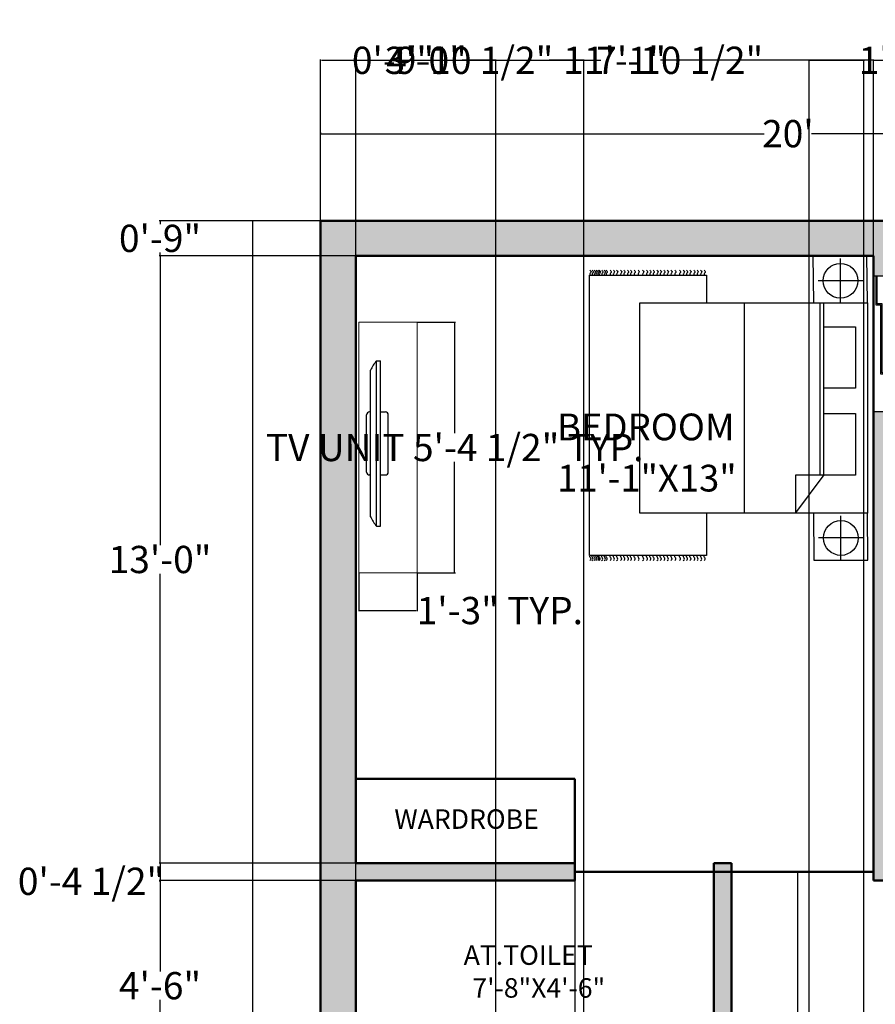
# Model space of a CAD drawing. Units: inches. Extents: x 48 to 822, y -191 to 651.
# Tile 7 of 13: x 48 to 268, y 398 to 651. Entities that reach past the tile are written whole.
import ezdxf

# ---------------------------------------------------------------- set-up
doc = ezdxf.new("R2010")
doc.units = ezdxf.units.IN
doc.header["$MEASUREMENT"] = 0
doc.layers.get('0').update_dxf_attribs({"color": 254})
for name, color, linetype, lineweight in [('A-ANNO-DIMS', 2, 'Continuous', 18), ('A-AREA-IDEN', 7, 'Continuous', 25), ('A-FURN', 8, 'Continuous', 18), ('A-GLAZ', 4, 'Continuous', 25), ('A-WALL', 7, 'Continuous', 50), ('A-WALL-PATT', 8, 'Continuous', 13)]:
    doc.layers.add(name, color=color, linetype=linetype, lineweight=lineweight)
doc.layers.add('furniture', color=250, linetype='Continuous')
doc.styles.get("Standard").update_dxf_attribs({"font": 'arial.ttf'})
doc.dimstyles.get("Standard").update_dxf_attribs({"dimtxt": 7, "dimasz": 0.18, "dimexe": 0.18, "dimexo": 0.0625, "dimgap": 0.09, "dimtad": 0, "dimtih": 1, "dimtoh": 1, "dimzin": 0, "dimdsep": 46, "dimlunit": 3, "dimtxsty": 'Standard', "dimcen": 0.09, "dimadec": 0, "dimazin": 0, "dimtfac": 1, "dimtofl": 0, "dimtmove": 0, "dimatfit": 3, "dimfxl": 1, "dimtolj": 1, "dimtzin": 0, "dimarcsym": 0})

# ---------------------------------------------------------------- blocks, each defined once
blk = doc.blocks.new('CARPET')
at = {"layer": 'furniture'}
for p, q in [((-51.53, -98.11), (-51.53, -55.12)), ((-51.53, -55.12), (-41.27, -55.12)), ((36, -55.12), (51.55, -55.12)), ((51.55, -55.12), (51.55, -98.11)), ((51.55, -98.11), (-51.53, -98.11))]:
    blk.add_line(p, q, dxfattribs=at)
for points, knots in [([(-53.37, -55.99), (-53.22, -55.8), (-52.9, -55.41), (-52.34, -55.8), (-51.89, -56.08), (-51.65, -55.91), (-51.53, -55.83)], [0, 0, 0, 0, 0.653278, 1.290138, 1.740457, 2.114451, 2.114451, 2.114451, 2.114451]), ([(-53.37, -57.26), (-53.22, -57.07), (-52.9, -56.67), (-52.34, -57.07), (-51.89, -57.35), (-51.65, -57.17), (-51.53, -57.1)], [0, 0, 0, 0, 0.653278, 1.290138, 1.740457, 2.114451, 2.114451, 2.114451, 2.114451]), ([(53.37, -55.99), (53.22, -55.8), (52.9, -55.41), (52.34, -55.8), (51.89, -56.08), (51.65, -55.91), (51.53, -55.83)], [0, 0, 0, 0, 0.653278, 1.290138, 1.740457, 2.114451, 2.114451, 2.114451, 2.114451]), ([(53.37, -57.26), (53.22, -57.07), (52.9, -56.67), (52.34, -57.07), (51.89, -57.35), (51.65, -57.17), (51.53, -57.1)], [0, 0, 0, 0, 0.653278, 1.290138, 1.740457, 2.114451, 2.114451, 2.114451, 2.114451]), ([(-53.37, -58.59), (-53.22, -58.4), (-52.9, -58.01), (-52.34, -58.4), (-51.89, -58.68), (-51.65, -58.5), (-51.53, -58.43)], [0, 0, 0, 0, 0.653278, 1.290138, 1.740457, 2.114451, 2.114451, 2.114451, 2.114451]), ([(-53.37, -59.78), (-53.22, -59.58), (-52.9, -59.19), (-52.34, -59.58), (-51.89, -59.86), (-51.65, -59.69), (-51.53, -59.61)], [0, 0, 0, 0, 0.653278, 1.290138, 1.740457, 2.114451, 2.114451, 2.114451, 2.114451]), ([(-53.37, -61.22), (-53.22, -61.02), (-52.9, -60.63), (-52.34, -61.02), (-51.89, -61.3), (-51.65, -61.13), (-51.53, -61.05)], [0, 0, 0, 0, 0.653278, 1.290138, 1.740457, 2.114451, 2.114451, 2.114451, 2.114451]), ([(53.37, -58.59), (53.22, -58.4), (52.9, -58.01), (52.34, -58.4), (51.89, -58.68), (51.65, -58.5), (51.53, -58.43)], [0, 0, 0, 0, 0.653278, 1.290138, 1.740457, 2.114451, 2.114451, 2.114451, 2.114451]), ([(53.37, -59.78), (53.22, -59.58), (52.9, -59.19), (52.34, -59.58), (51.89, -59.86), (51.65, -59.69), (51.53, -59.61)], [0, 0, 0, 0, 0.653278, 1.290138, 1.740457, 2.114451, 2.114451, 2.114451, 2.114451]), ([(53.37, -61.22), (53.22, -61.02), (52.9, -60.63), (52.34, -61.02), (51.89, -61.3), (51.65, -61.13), (51.53, -61.05)], [0, 0, 0, 0, 0.653278, 1.290138, 1.740457, 2.114451, 2.114451, 2.114451, 2.114451]), ([(-53.37, -62.44), (-53.22, -62.25), (-52.9, -61.86), (-52.34, -62.25), (-51.89, -62.53), (-51.65, -62.36), (-51.53, -62.28)], [0, 0, 0, 0, 0.653278, 1.290138, 1.740457, 2.114451, 2.114451, 2.114451, 2.114451]), ([(-53.37, -63.63), (-53.22, -63.43), (-52.9, -63.04), (-52.34, -63.43), (-51.89, -63.72), (-51.65, -63.54), (-51.53, -63.46)], [0, 0, 0, 0, 0.653278, 1.290138, 1.740457, 2.114451, 2.114451, 2.114451, 2.114451]), ([(-53.37, -65.07), (-53.22, -64.87), (-52.9, -64.48), (-52.34, -64.87), (-51.89, -65.15), (-51.65, -64.98), (-51.53, -64.9)], [0, 0, 0, 0, 0.653278, 1.290138, 1.740457, 2.114451, 2.114451, 2.114451, 2.114451]), ([(53.37, -62.44), (53.22, -62.25), (52.9, -61.86), (52.34, -62.25), (51.89, -62.53), (51.65, -62.36), (51.53, -62.28)], [0, 0, 0, 0, 0.653278, 1.290138, 1.740457, 2.114451, 2.114451, 2.114451, 2.114451]), ([(53.37, -63.63), (53.22, -63.43), (52.9, -63.04), (52.34, -63.43), (51.89, -63.72), (51.65, -63.54), (51.53, -63.46)], [0, 0, 0, 0, 0.653278, 1.290138, 1.740457, 2.114451, 2.114451, 2.114451, 2.114451]), ([(53.37, -65.07), (53.22, -64.87), (52.9, -64.48), (52.34, -64.87), (51.89, -65.15), (51.65, -64.98), (51.53, -64.9)], [0, 0, 0, 0, 0.653278, 1.290138, 1.740457, 2.114451, 2.114451, 2.114451, 2.114451]), ([(-53.37, -66.76), (-53.22, -66.56), (-52.9, -66.17), (-52.34, -66.56), (-51.89, -66.84), (-51.65, -66.67), (-51.53, -66.59)], [0, 0, 0, 0, 0.653278, 1.290138, 1.740457, 2.114451, 2.114451, 2.114451, 2.114451]), ([(-53.37, -68.2), (-53.22, -68), (-52.9, -67.61), (-52.34, -68), (-51.89, -68.28), (-51.65, -68.11), (-51.53, -68.03)], [0, 0, 0, 0, 0.653278, 1.290138, 1.740457, 2.114451, 2.114451, 2.114451, 2.114451]), ([(53.37, -66.76), (53.22, -66.56), (52.9, -66.17), (52.34, -66.56), (51.89, -66.84), (51.65, -66.67), (51.53, -66.59)], [0, 0, 0, 0, 0.653278, 1.290138, 1.740457, 2.114451, 2.114451, 2.114451, 2.114451]), ([(53.37, -68.2), (53.22, -68), (52.9, -67.61), (52.34, -68), (51.89, -68.28), (51.65, -68.11), (51.53, -68.03)], [0, 0, 0, 0, 0.653278, 1.290138, 1.740457, 2.114451, 2.114451, 2.114451, 2.114451]), ([(-53.37, -69.53), (-53.22, -69.33), (-52.9, -68.94), (-52.34, -69.33), (-51.89, -69.61), (-51.65, -69.44), (-51.53, -69.36)], [0, 0, 0, 0, 0.653278, 1.290138, 1.740457, 2.114451, 2.114451, 2.114451, 2.114451]), ([(-53.37, -70.79), (-53.22, -70.6), (-52.9, -70.21), (-52.34, -70.6), (-51.89, -70.88), (-51.65, -70.7), (-51.53, -70.63)], [0, 0, 0, 0, 0.653278, 1.290138, 1.740457, 2.114451, 2.114451, 2.114451, 2.114451]), ([(-53.37, -72.12), (-53.22, -71.93), (-52.9, -71.54), (-52.34, -71.93), (-51.89, -72.21), (-51.65, -72.04), (-51.53, -71.96)], [0, 0, 0, 0, 0.653278, 1.290138, 1.740457, 2.114451, 2.114451, 2.114451, 2.114451]), ([(53.37, -69.53), (53.22, -69.33), (52.9, -68.94), (52.34, -69.33), (51.89, -69.61), (51.65, -69.44), (51.53, -69.36)], [0, 0, 0, 0, 0.653278, 1.290138, 1.740457, 2.114451, 2.114451, 2.114451, 2.114451]), ([(53.37, -70.79), (53.22, -70.6), (52.9, -70.21), (52.34, -70.6), (51.89, -70.88), (51.65, -70.7), (51.53, -70.63)], [0, 0, 0, 0, 0.653278, 1.290138, 1.740457, 2.114451, 2.114451, 2.114451, 2.114451]), ([(53.37, -72.12), (53.22, -71.93), (52.9, -71.54), (52.34, -71.93), (51.89, -72.21), (51.65, -72.04), (51.53, -71.96)], [0, 0, 0, 0, 0.653278, 1.290138, 1.740457, 2.114451, 2.114451, 2.114451, 2.114451]), ([(-53.37, -73.31), (-53.22, -73.11), (-52.9, -72.72), (-52.34, -73.11), (-51.89, -73.4), (-51.65, -73.22), (-51.53, -73.14)], [0, 0, 0, 0, 0.653278, 1.290138, 1.740457, 2.114451, 2.114451, 2.114451, 2.114451]), ([(-53.37, -74.75), (-53.22, -74.55), (-52.9, -74.16), (-52.34, -74.55), (-51.89, -74.83), (-51.65, -74.66), (-51.53, -74.58)], [0, 0, 0, 0, 0.653278, 1.290138, 1.740457, 2.114451, 2.114451, 2.114451, 2.114451]), ([(-53.37, -75.98), (-53.22, -75.78), (-52.9, -75.39), (-52.34, -75.78), (-51.89, -76.06), (-51.65, -75.89), (-51.53, -75.81)], [0, 0, 0, 0, 0.653278, 1.290138, 1.740457, 2.114451, 2.114451, 2.114451, 2.114451]), ([(53.37, -73.31), (53.22, -73.11), (52.9, -72.72), (52.34, -73.11), (51.89, -73.4), (51.65, -73.22), (51.53, -73.14)], [0, 0, 0, 0, 0.653278, 1.290138, 1.740457, 2.114451, 2.114451, 2.114451, 2.114451]), ([(53.37, -74.75), (53.22, -74.55), (52.9, -74.16), (52.34, -74.55), (51.89, -74.83), (51.65, -74.66), (51.53, -74.58)], [0, 0, 0, 0, 0.653278, 1.290138, 1.740457, 2.114451, 2.114451, 2.114451, 2.114451]), ([(53.37, -75.98), (53.22, -75.78), (52.9, -75.39), (52.34, -75.78), (51.89, -76.06), (51.65, -75.89), (51.53, -75.81)], [0, 0, 0, 0, 0.653278, 1.290138, 1.740457, 2.114451, 2.114451, 2.114451, 2.114451]), ([(-53.37, -77.16), (-53.22, -76.96), (-52.9, -76.57), (-52.34, -76.96), (-51.89, -77.25), (-51.65, -77.07), (-51.53, -76.99)], [0, 0, 0, 0, 0.653278, 1.290138, 1.740457, 2.114451, 2.114451, 2.114451, 2.114451]), ([(-53.37, -78.6), (-53.22, -78.4), (-52.9, -78.01), (-52.34, -78.4), (-51.89, -78.68), (-51.65, -78.51), (-51.53, -78.43)], [0, 0, 0, 0, 0.653278, 1.290138, 1.740457, 2.114451, 2.114451, 2.114451, 2.114451]), ([(53.37, -77.16), (53.22, -76.96), (52.9, -76.57), (52.34, -76.96), (51.89, -77.25), (51.65, -77.07), (51.53, -76.99)], [0, 0, 0, 0, 0.653278, 1.290138, 1.740457, 2.114451, 2.114451, 2.114451, 2.114451]), ([(53.37, -78.6), (53.22, -78.4), (52.9, -78.01), (52.34, -78.4), (51.89, -78.68), (51.65, -78.51), (51.53, -78.43)], [0, 0, 0, 0, 0.653278, 1.290138, 1.740457, 2.114451, 2.114451, 2.114451, 2.114451]), ([(-53.37, -80.29), (-53.22, -80.09), (-52.9, -79.7), (-52.34, -80.09), (-51.89, -80.37), (-51.65, -80.2), (-51.53, -80.12)], [0, 0, 0, 0, 0.653278, 1.290138, 1.740457, 2.114451, 2.114451, 2.114451, 2.114451]), ([(-53.37, -81.73), (-53.22, -81.53), (-52.9, -81.14), (-52.34, -81.53), (-51.89, -81.81), (-51.65, -81.64), (-51.53, -81.56)], [0, 0, 0, 0, 0.653278, 1.290138, 1.740457, 2.114451, 2.114451, 2.114451, 2.114451]), ([(-53.37, -83.06), (-53.22, -82.86), (-52.9, -82.47), (-52.34, -82.86), (-51.89, -83.14), (-51.65, -82.97), (-51.53, -82.89)], [0, 0, 0, 0, 0.653278, 1.290138, 1.740457, 2.114451, 2.114451, 2.114451, 2.114451]), ([(53.37, -80.29), (53.22, -80.09), (52.9, -79.7), (52.34, -80.09), (51.89, -80.37), (51.65, -80.2), (51.53, -80.12)], [0, 0, 0, 0, 0.653278, 1.290138, 1.740457, 2.114451, 2.114451, 2.114451, 2.114451]), ([(53.37, -81.73), (53.22, -81.53), (52.9, -81.14), (52.34, -81.53), (51.89, -81.81), (51.65, -81.64), (51.53, -81.56)], [0, 0, 0, 0, 0.653278, 1.290138, 1.740457, 2.114451, 2.114451, 2.114451, 2.114451]), ([(53.37, -83.06), (53.22, -82.86), (52.9, -82.47), (52.34, -82.86), (51.89, -83.14), (51.65, -82.97), (51.53, -82.89)], [0, 0, 0, 0, 0.653278, 1.290138, 1.740457, 2.114451, 2.114451, 2.114451, 2.114451]), ([(-53.37, -84.18), (-53.22, -83.99), (-52.9, -83.6), (-52.34, -83.99), (-51.89, -84.27), (-51.65, -84.09), (-51.53, -84.02)], [0, 0, 0, 0, 0.653278, 1.290138, 1.740457, 2.114451, 2.114451, 2.114451, 2.114451]), ([(-53.37, -85.51), (-53.22, -85.32), (-52.9, -84.93), (-52.34, -85.32), (-51.89, -85.6), (-51.65, -85.42), (-51.53, -85.35)], [0, 0, 0, 0, 0.653278, 1.290138, 1.740457, 2.114451, 2.114451, 2.114451, 2.114451]), ([(-53.37, -86.7), (-53.22, -86.5), (-52.9, -86.11), (-52.34, -86.5), (-51.89, -86.78), (-51.65, -86.61), (-51.53, -86.53)], [0, 0, 0, 0, 0.653278, 1.290138, 1.740457, 2.114451, 2.114451, 2.114451, 2.114451]), ([(53.37, -84.18), (53.22, -83.99), (52.9, -83.6), (52.34, -83.99), (51.89, -84.27), (51.65, -84.09), (51.53, -84.02)], [0, 0, 0, 0, 0.653278, 1.290138, 1.740457, 2.114451, 2.114451, 2.114451, 2.114451]), ([(53.37, -85.51), (53.22, -85.32), (52.9, -84.93), (52.34, -85.32), (51.89, -85.6), (51.65, -85.42), (51.53, -85.35)], [0, 0, 0, 0, 0.653278, 1.290138, 1.740457, 2.114451, 2.114451, 2.114451, 2.114451]), ([(53.37, -86.7), (53.22, -86.5), (52.9, -86.11), (52.34, -86.5), (51.89, -86.78), (51.65, -86.61), (51.53, -86.53)], [0, 0, 0, 0, 0.653278, 1.290138, 1.740457, 2.114451, 2.114451, 2.114451, 2.114451]), ([(-53.37, -88.14), (-53.22, -87.94), (-52.9, -87.55), (-52.34, -87.94), (-51.89, -88.22), (-51.65, -88.05), (-51.53, -87.97)], [0, 0, 0, 0, 0.653278, 1.290138, 1.740457, 2.114451, 2.114451, 2.114451, 2.114451]), ([(-53.37, -89.36), (-53.22, -89.17), (-52.9, -88.78), (-52.34, -89.17), (-51.89, -89.45), (-51.65, -89.28), (-51.53, -89.2)], [0, 0, 0, 0, 0.653278, 1.290138, 1.740457, 2.114451, 2.114451, 2.114451, 2.114451]), ([(-53.37, -90.55), (-53.22, -90.35), (-52.9, -89.96), (-52.34, -90.35), (-51.89, -90.64), (-51.65, -90.46), (-51.53, -90.38)], [0, 0, 0, 0, 0.653278, 1.290138, 1.740457, 2.114451, 2.114451, 2.114451, 2.114451]), ([(53.37, -88.14), (53.22, -87.94), (52.9, -87.55), (52.34, -87.94), (51.89, -88.22), (51.65, -88.05), (51.53, -87.97)], [0, 0, 0, 0, 0.653278, 1.290138, 1.740457, 2.114451, 2.114451, 2.114451, 2.114451]), ([(53.37, -89.36), (53.22, -89.17), (52.9, -88.78), (52.34, -89.17), (51.89, -89.45), (51.65, -89.28), (51.53, -89.2)], [0, 0, 0, 0, 0.653278, 1.290138, 1.740457, 2.114451, 2.114451, 2.114451, 2.114451]), ([(53.37, -90.55), (53.22, -90.35), (52.9, -89.96), (52.34, -90.35), (51.9, -90.63), (51.66, -90.47), (51.55, -90.4)], [0, 0, 0, 0, 0.653278, 1.290138, 1.740457, 2.0926, 2.0926, 2.0926, 2.0926]), ([(-53.37, -91.99), (-53.22, -91.79), (-52.9, -91.4), (-52.34, -91.79), (-51.89, -92.07), (-51.65, -91.9), (-51.53, -91.82)], [0, 0, 0, 0, 0.653278, 1.290138, 1.740457, 2.114451, 2.114451, 2.114451, 2.114451]), ([(-53.37, -92.69), (-53.22, -92.48), (-52.9, -92.08), (-52.35, -92.49), (-51.89, -92.77), (-51.65, -92.6), (-51.53, -92.52)], [0, 0, 0, 0, 0.663904, 1.307406, 1.757725, 2.131719, 2.131719, 2.131719, 2.131719]), ([(-53.37, -93.61), (-53.22, -93.42), (-52.9, -93.03), (-52.34, -93.42), (-51.89, -93.7), (-51.65, -93.52), (-51.53, -93.45)], [0, 0, 0, 0, 0.653278, 1.290138, 1.740457, 2.114451, 2.114451, 2.114451, 2.114451]), ([(-53.37, -94.55), (-53.22, -94.35), (-52.9, -93.96), (-52.34, -94.35), (-51.89, -94.63), (-51.65, -94.46), (-51.53, -94.38)], [0, 0, 0, 0, 0.653278, 1.290138, 1.740457, 2.114451, 2.114451, 2.114451, 2.114451]), ([(53.37, -91.99), (53.22, -91.79), (52.9, -91.4), (52.34, -91.79), (51.9, -92.07), (51.66, -91.91), (51.55, -91.83)], [0, 0, 0, 0, 0.653278, 1.290138, 1.740457, 2.0926, 2.0926, 2.0926, 2.0926]), ([(53.37, -92.69), (53.22, -92.49), (52.9, -92.09), (52.34, -92.49), (51.9, -92.77), (51.66, -92.61), (51.55, -92.53)], [0, 0, 0, 0, 0.656792, 1.295826, 1.746145, 2.098292, 2.098292, 2.098292, 2.098292]), ([(53.37, -93.66), (53.22, -93.46), (52.9, -93.07), (52.34, -93.46), (51.9, -93.74), (51.66, -93.58), (51.55, -93.5)], [0, 0, 0, 0, 0.653278, 1.290138, 1.740457, 2.0926, 2.0926, 2.0926, 2.0926]), ([(53.37, -94.59), (53.22, -94.4), (52.9, -94.01), (52.34, -94.4), (51.9, -94.68), (51.66, -94.51), (51.55, -94.44)], [0, 0, 0, 0, 0.653278, 1.290138, 1.740457, 2.0926, 2.0926, 2.0926, 2.0926]), ([(-53.37, -95.05), (-53.22, -94.85), (-52.9, -94.46), (-52.34, -94.85), (-51.89, -95.14), (-51.65, -94.96), (-51.53, -94.88)], [0, 0, 0, 0, 0.653278, 1.290138, 1.740457, 2.114451, 2.114451, 2.114451, 2.114451]), ([(-53.37, -95.73), (-53.22, -95.54), (-52.9, -95.15), (-52.34, -95.54), (-51.89, -95.82), (-51.65, -95.65), (-51.53, -95.57)], [0, 0, 0, 0, 0.653278, 1.290138, 1.740457, 2.114451, 2.114451, 2.114451, 2.114451]), ([(-53.37, -96.38), (-53.22, -96.18), (-52.9, -95.79), (-52.34, -96.18), (-51.89, -96.47), (-51.65, -96.29), (-51.53, -96.21)], [0, 0, 0, 0, 0.653278, 1.290138, 1.740457, 2.114451, 2.114451, 2.114451, 2.114451]), ([(-53.37, -97.17), (-53.22, -96.98), (-52.9, -96.59), (-52.34, -96.98), (-51.89, -97.26), (-51.65, -97.08), (-51.53, -97.01)], [0, 0, 0, 0, 0.653278, 1.290138, 1.740457, 2.114451, 2.114451, 2.114451, 2.114451]), ([(-53.37, -97.99), (-53.22, -97.79), (-52.9, -97.4), (-52.34, -97.79), (-51.89, -98.08), (-51.65, -97.9), (-51.53, -97.82)], [0, 0, 0, 0, 0.653278, 1.290138, 1.740457, 2.114451, 2.114451, 2.114451, 2.114451]), ([(53.37, -95.78), (53.22, -95.58), (52.9, -95.19), (52.34, -95.58), (51.89, -95.86), (51.65, -95.69), (51.53, -95.61)], [0, 0, 0, 0, 0.653278, 1.290138, 1.740457, 2.114451, 2.114451, 2.114451, 2.114451]), ([(53.37, -96.43), (53.22, -96.23), (52.9, -95.84), (52.34, -96.23), (51.89, -96.51), (51.65, -96.34), (51.53, -96.26)], [0, 0, 0, 0, 0.653278, 1.290138, 1.740457, 2.114451, 2.114451, 2.114451, 2.114451]), ([(53.37, -97.22), (53.22, -97.02), (52.9, -96.63), (52.34, -97.02), (51.89, -97.3), (51.65, -97.13), (51.53, -97.05)], [0, 0, 0, 0, 0.653278, 1.290138, 1.740457, 2.114451, 2.114451, 2.114451, 2.114451]), ([(53.37, -97.99), (53.22, -97.79), (52.9, -97.4), (52.34, -97.79), (51.89, -98.08), (51.65, -97.9), (51.53, -97.82)], [0, 0, 0, 0, 0.653278, 1.290138, 1.740457, 2.114451, 2.114451, 2.114451, 2.114451]), ([(53.37, -95.1), (53.22, -94.9), (52.9, -94.51), (52.34, -94.9), (51.9, -95.18), (51.66, -95.02), (51.55, -94.94)], [0, 0, 0, 0, 0.653278, 1.290138, 1.740457, 2.0926, 2.0926, 2.0926, 2.0926])]:
    blk.add_open_spline(points, degree=3, knots=knots, dxfattribs=at)
blk = doc.blocks.new('A$C58D270C6')
at = {"layer": 'furniture'}
for p, q in [((9.09, 124.13), (9.09, 108.87)), ((1.46, 116.5), (16.73, 116.5)), ((42.08, 108), (42.08, 36)), ((14.97, 94.84), (24.62, 107.92)), ((24.62, 94.93), (24.62, 107.92)), ((14.97, 94.93), (24.62, 94.93)), ((14.97, 94.84), (14.97, 36)), ((16.22, 94.93), (16.22, 36)), ((9.25, 36), (9.25, 20.74)), ((1.62, 28.37), (16.88, 28.37))]:
    blk.add_line(p, q, dxfattribs=at)
for points in [[(18.5, 108), (18.34, 124.13), (-0.16, 124.13), (0, 108)], [(0, 108), (77.91, 108), (77.91, 36), (0, 36)], [(4.09, 94.93), (14.97, 94.93), (14.97, 73.83), (4.09, 73.83)], [(4.09, 65.23), (14.97, 65.23), (14.97, 44.13), (4.09, 44.13)], [(18.65, 19.87), (18.5, 36), (0, 36), (0.16, 19.87)]]:
    blk.add_lwpolyline(points, close=True, dxfattribs=at)
for centre in [(9.09, 116.5), (9.25, 28.37)]:
    blk.add_circle(centre, 5.95, dxfattribs=at)
at = {"layer": 'furniture', "xscale": 0.9312884925094044, "yscale": 0.9312884925094044, "zscale": 0.9312884925094044, "rotation": 90}
blk.add_blockref('CARPET', (3.79, 74.47), dxfattribs=at)
blk = doc.blocks.new('PLASMA-LARGE')
at = {"layer": 'furniture'}
for p, q in [((-7.26, 0), (7.26, 0)), ((-21, -2.5), (21, -2.5)), ((-21, -2.5), (-21, -3.5)), ((-18.61, -1), (18.61, -1)), ((-8, -1), (-8, -0.74)), ((8, -1), (8, -0.74)), ((21, -2.5), (21, -3.5)), ((-21, -3.5), (21, -3.5)), ((-8, -3.5), (-8, -4.76)), ((8, -3.5), (8, -4.76)), ((-7.26, -5.5), (7.26, -5.5))]:
    blk.add_line(p, q, dxfattribs=at)
for centre, radius, start, end in [((-7.26, -0.74), 0.744, 90, 180), ((7.26, -0.74), 0.744, 0, 90), ((-13.97, -11.05), 11.07, 114.7602, 129.4175), ((13.97, -11.05), 11.07, 50.5825, 65.2398), ((-7.26, -4.76), 0.744, 180, 270), ((7.26, -4.76), 0.744, 270, 0)]:
    blk.add_arc(centre, radius, start, end, dxfattribs=at)
blk = doc.blocks.new('*D16')
at = {"layer": 'A-ANNO-DIMS', "color": 0, "lineweight": -2, "transparency": 16777216}
for p, q in [((125.45, 622.39), (125.45, 621.91)), ((365.45, 622.39), (365.45, 621.91)), ((125.63, 622.09), (239.36, 622.09)), ((365.27, 622.09), (251.54, 622.09))]:
    blk.add_line(p, q, dxfattribs=at)
at = {"layer": 'A-ANNO-DIMS', "color": 0, "transparency": 16777216}
for points in [[(125.63, 622.12), (125.63, 622.06), (125.45, 622.09)], [(365.27, 622.12), (365.27, 622.06), (365.45, 622.09)]]:
    blk.add_solid(points, dxfattribs=at)
at = {"layer": 'Defpoints', "color": 0, "transparency": 16777216}
for p in [(125.45, 622.45), (365.45, 622.45), (365.45, 622.09)]:
    blk.add_point(p, dxfattribs=at)
at = {"layer": 'A-ANNO-DIMS', "color": 0, "transparency": 16777216, "insert": (245.45, 622.09), "char_height": 7, "attachment_point": 5}
blk.add_mtext("\\A1;20'", dxfattribs=at)
blk = doc.blocks.new('*D17')
at = {"layer": 'A-ANNO-DIMS', "color": 0, "lineweight": -2, "transparency": 16777216}
for p, q in [((109.06, 599.69), (107.79, 599.69)), ((107.97, 599.51), (107.97, 243.35)), ((107.97, -120.13), (107.97, 236.02)), ((109.06, -120.31), (107.79, -120.31))]:
    blk.add_line(p, q, dxfattribs=at)
at = {"layer": 'A-ANNO-DIMS', "color": 0, "transparency": 16777216}
for points in [[(107.94, 599.51), (108, 599.51), (107.97, 599.69)], [(107.94, -120.13), (108, -120.13), (107.97, -120.31)]]:
    blk.add_solid(points, dxfattribs=at)
at = {"layer": 'Defpoints', "color": 0, "transparency": 16777216}
for p in [(109.12, 599.69), (107.97, -120.31), (109.12, -120.31)]:
    blk.add_point(p, dxfattribs=at)
at = {"layer": 'A-ANNO-DIMS', "color": 0, "transparency": 16777216, "insert": (107.97, 239.69), "char_height": 7, "attachment_point": 5}
blk.add_mtext("\\A1;60'", dxfattribs=at)
blk = doc.blocks.new('*D20')
at = {"layer": 'A-ANNO-DIMS', "color": 0, "lineweight": -2, "transparency": 16777216}
for p, q in [((247.94, 432.26), (247.94, 367.48)), ((248, 432.44), (248.12, 432.44)), ((247.94, 295.37), (247.94, 360.15)), ((248, 295.19), (248.12, 295.19))]:
    blk.add_line(p, q, dxfattribs=at)
at = {"layer": 'A-ANNO-DIMS', "color": 0, "transparency": 16777216}
for points in [[(247.91, 432.26), (247.97, 432.26), (247.94, 432.44)], [(247.91, 295.37), (247.97, 295.37), (247.94, 295.19)]]:
    blk.add_solid(points, dxfattribs=at)
at = {"layer": 'Defpoints', "color": 0, "transparency": 16777216}
for p in [(247.94, 432.44), (247.94, 432.44), (247.94, 295.19)]:
    blk.add_point(p, dxfattribs=at)
at = {"layer": 'A-ANNO-DIMS', "color": 0, "transparency": 16777216, "insert": (247.94, 363.81), "char_height": 7, "attachment_point": 5}
blk.add_mtext('\\A1;11\'-5.25"', dxfattribs=at)
blk = doc.blocks.new('WIN-900-SLIT')
for p, q in [((271.95, 585.52), (267.45, 585.52)), ((267.45, 585.52), (267.45, 550.72)), ((268.05, 585.52), (268.05, 578.13)), ((268.38, 578.41), (268.38, 585.52)), ((271.95, 550.72), (271.95, 585.52)), ((268.05, 578.13), (269.28, 578.13)), ((269.63, 578.41), (268.38, 578.41)), ((269.28, 578.13), (269.28, 560.35)), ((269.63, 560.61), (269.63, 578.41)), ((269.28, 560.35), (270.46, 560.35)), ((270.92, 560.61), (269.63, 560.61)), ((270.46, 560.35), (270.46, 550.72)), ((270.92, 550.72), (270.92, 560.61)), ((267.45, 550.72), (271.95, 550.72))]:
    blk.add_line(p, q)
blk = doc.blocks.new('TV-UNIT')
for p, q in [((14.9, 64.44), (0, 64.44)), ((0, 64.44), (0, 0)), ((14.9, 64.44), (14.9, 0)), ((0, 0), (14.9, 0))]:
    blk.add_line(p, q)
blk = doc.blocks.new('*D38')
at = {"layer": 'A-ANNO-DIMS', "color": 0, "lineweight": -2, "transparency": 16777216}
for p, q in [((150.26, 573.68), (160.05, 573.68)), ((159.87, 573.5), (159.87, 545.17)), ((159.87, 509.42), (159.87, 537.75)), ((150.26, 509.24), (160.05, 509.24))]:
    blk.add_line(p, q, dxfattribs=at)
at = {"layer": 'A-ANNO-DIMS', "color": 0, "transparency": 16777216}
for points in [[(159.84, 573.5), (159.9, 573.5), (159.87, 573.68)], [(159.84, 509.42), (159.9, 509.42), (159.87, 509.24)]]:
    blk.add_solid(points, dxfattribs=at)
at = {"layer": 'Defpoints', "color": 0, "transparency": 16777216}
for p in [(150.2, 573.68), (159.87, 573.68), (150.2, 509.24)]:
    blk.add_point(p, dxfattribs=at)
at = {"layer": 'A-ANNO-DIMS', "color": 0, "transparency": 16777216, "insert": (159.87, 541.46), "char_height": 7, "attachment_point": 5}
blk.add_mtext('\\A1;TV UNIT 5\'-4 1/2" TYP.', dxfattribs=at)
blk = doc.blocks.new('*D39')
at = {"layer": 'A-ANNO-DIMS', "color": 0, "lineweight": -2, "transparency": 16777216}
for p, q in [((135.3, 509.17), (135.3, 499.39)), ((150.2, 509.17), (150.2, 499.39)), ((135.48, 499.57), (150.02, 499.57)), ((150.2, 499.57), (150.38, 499.57))]:
    blk.add_line(p, q, dxfattribs=at)
at = {"layer": 'A-ANNO-DIMS', "color": 0, "transparency": 16777216}
for points in [[(135.48, 499.6), (135.48, 499.54), (135.3, 499.57)], [(150.02, 499.6), (150.02, 499.54), (150.2, 499.57)]]:
    blk.add_solid(points, dxfattribs=at)
at = {"layer": 'Defpoints', "color": 0, "transparency": 16777216}
for p in [(135.3, 509.24), (150.2, 509.24), (150.2, 499.57)]:
    blk.add_point(p, dxfattribs=at)
at = {"layer": 'A-ANNO-DIMS', "color": 0, "transparency": 16777216, "insert": (171.47, 499.57), "char_height": 7, "attachment_point": 5}
blk.add_mtext('\\A1;1\'-3" TYP.', dxfattribs=at)
blk = doc.blocks.new('*D60')
at = {"layer": 'A-ANNO-DIMS', "color": 0, "lineweight": -2, "transparency": 16777216}
for p, q in [((125.45, 599.75), (125.45, 641.12)), ((125.63, 640.94), (134.27, 640.94)), ((134.45, 590.75), (134.45, 641.12)), ((134.45, 640.94), (134.63, 640.94))]:
    blk.add_line(p, q, dxfattribs=at)
at = {"layer": 'A-ANNO-DIMS', "color": 0, "transparency": 16777216}
for points in [[(125.63, 640.97), (125.63, 640.91), (125.45, 640.94)], [(134.27, 640.97), (134.27, 640.91), (134.45, 640.94)]]:
    blk.add_solid(points, dxfattribs=at)
at = {"layer": 'Defpoints', "color": 0, "transparency": 16777216}
for p in [(134.45, 640.94), (125.45, 599.69), (134.45, 590.69)]:
    blk.add_point(p, dxfattribs=at)
at = {"layer": 'A-ANNO-DIMS', "color": 0, "transparency": 16777216, "insert": (144.02, 640.94), "char_height": 7, "attachment_point": 5}
blk.add_mtext('\\A1;0\'-9"', dxfattribs=at)
blk = doc.blocks.new('*D61')
at = {"layer": 'A-ANNO-DIMS', "color": 0, "lineweight": -2, "transparency": 16777216}
for p, q in [((134.45, 590.75), (134.45, 641.12)), ((134.63, 640.94), (189.17, 640.94)), ((267.27, 640.94), (212.73, 640.94)), ((267.45, 590.75), (267.45, 641.12))]:
    blk.add_line(p, q, dxfattribs=at)
at = {"layer": 'A-ANNO-DIMS', "color": 0, "transparency": 16777216}
for points in [[(134.63, 640.97), (134.63, 640.91), (134.45, 640.94)], [(267.27, 640.97), (267.27, 640.91), (267.45, 640.94)]]:
    blk.add_solid(points, dxfattribs=at)
at = {"layer": 'Defpoints', "color": 0, "transparency": 16777216}
for p in [(267.45, 640.94), (134.45, 590.69), (267.45, 590.69)]:
    blk.add_point(p, dxfattribs=at)
at = {"layer": 'A-ANNO-DIMS', "color": 0, "transparency": 16777216, "insert": (200.95, 640.94), "char_height": 7, "attachment_point": 5}
blk.add_mtext('\\A1;11\'-1"', dxfattribs=at)
blk = doc.blocks.new('*D62')
at = {"layer": 'A-ANNO-DIMS', "color": 0, "lineweight": -2, "transparency": 16777216}
for p, q in [((267.45, 590.75), (267.45, 641.12)), ((267.63, 640.94), (271.77, 640.94)), ((271.95, 590.75), (271.95, 641.12)), ((271.95, 640.94), (272.13, 640.94))]:
    blk.add_line(p, q, dxfattribs=at)
at = {"layer": 'A-ANNO-DIMS', "color": 0, "transparency": 16777216}
for points in [[(267.63, 640.97), (267.63, 640.91), (267.45, 640.94)], [(271.77, 640.97), (271.77, 640.91), (271.95, 640.94)]]:
    blk.add_solid(points, dxfattribs=at)
at = {"layer": 'Defpoints', "color": 0, "transparency": 16777216}
for p in [(271.95, 640.94), (267.45, 590.69), (271.95, 590.69)]:
    blk.add_point(p, dxfattribs=at)
at = {"layer": 'A-ANNO-DIMS', "color": 0, "transparency": 16777216, "insert": (289.68, 640.94), "char_height": 7, "attachment_point": 5}
blk.add_mtext('\\A1;0\'-4 1/2"', dxfattribs=at)
blk = doc.blocks.new('*D70')
at = {"layer": 'A-ANNO-DIMS', "color": 0, "lineweight": -2, "transparency": 16777216}
for p, q in [((125.39, 599.69), (84.02, 599.69)), ((84.2, 599.51), (84.2, 598.85)), ((134.39, 590.69), (84.02, 590.69)), ((84.2, 590.87), (84.2, 591.52))]:
    blk.add_line(p, q, dxfattribs=at)
at = {"layer": 'A-ANNO-DIMS', "color": 0, "transparency": 16777216}
for points in [[(84.17, 599.51), (84.23, 599.51), (84.2, 599.69)], [(84.17, 590.87), (84.23, 590.87), (84.2, 590.69)]]:
    blk.add_solid(points, dxfattribs=at)
at = {"layer": 'Defpoints', "color": 0, "transparency": 16777216}
for p in [(125.45, 599.69), (84.2, 590.69), (134.45, 590.69)]:
    blk.add_point(p, dxfattribs=at)
at = {"layer": 'A-ANNO-DIMS', "color": 0, "transparency": 16777216, "insert": (84.2, 595.19), "char_height": 7, "attachment_point": 5}
blk.add_mtext('\\A1;0\'-9"', dxfattribs=at)
blk = doc.blocks.new('*D71')
at = {"layer": 'A-ANNO-DIMS', "color": 0, "lineweight": -2, "transparency": 16777216}
for p, q in [((134.39, 590.69), (84.02, 590.69)), ((84.2, 590.51), (84.2, 516.35)), ((84.2, 434.87), (84.2, 509.02)), ((134.39, 434.69), (84.02, 434.69))]:
    blk.add_line(p, q, dxfattribs=at)
at = {"layer": 'A-ANNO-DIMS', "color": 0, "transparency": 16777216}
for points in [[(84.17, 590.51), (84.23, 590.51), (84.2, 590.69)], [(84.17, 434.87), (84.23, 434.87), (84.2, 434.69)]]:
    blk.add_solid(points, dxfattribs=at)
at = {"layer": 'Defpoints', "color": 0, "transparency": 16777216}
for p in [(134.45, 590.69), (84.2, 434.69), (134.45, 434.69)]:
    blk.add_point(p, dxfattribs=at)
at = {"layer": 'A-ANNO-DIMS', "color": 0, "transparency": 16777216, "insert": (84.2, 512.69), "char_height": 7, "attachment_point": 5}
blk.add_mtext('\\A1;13\'-0"', dxfattribs=at)
blk = doc.blocks.new('*D72')
at = {"layer": 'A-ANNO-DIMS', "color": 0, "lineweight": -2, "transparency": 16777216}
for p, q in [((134.39, 434.69), (84.02, 434.69)), ((84.2, 434.51), (84.2, 430.37)), ((134.39, 430.19), (84.02, 430.19)), ((84.2, 430.19), (84.2, 430.01)), ((84.2, 430.01), (84.02, 430.01))]:
    blk.add_line(p, q, dxfattribs=at)
at = {"layer": 'A-ANNO-DIMS', "color": 0, "transparency": 16777216}
for points in [[(84.17, 434.51), (84.23, 434.51), (84.2, 434.69)], [(84.17, 430.37), (84.23, 430.37), (84.2, 430.19)]]:
    blk.add_solid(points, dxfattribs=at)
at = {"layer": 'Defpoints', "color": 0, "transparency": 16777216}
for p in [(134.45, 434.69), (84.2, 430.19), (134.45, 430.19)]:
    blk.add_point(p, dxfattribs=at)
at = {"layer": 'A-ANNO-DIMS', "color": 0, "transparency": 16777216, "insert": (66.47, 430.01), "char_height": 7, "attachment_point": 5}
blk.add_mtext('\\A1;0\'-4 1/2"', dxfattribs=at)
blk = doc.blocks.new('*D73')
at = {"layer": 'A-ANNO-DIMS', "color": 0, "lineweight": -2, "transparency": 16777216}
for p, q in [((134.39, 430.19), (84.02, 430.19)), ((84.2, 430.01), (84.2, 406.85)), ((84.2, 376.37), (84.2, 399.52)), ((134.39, 376.19), (84.02, 376.19))]:
    blk.add_line(p, q, dxfattribs=at)
at = {"layer": 'A-ANNO-DIMS', "color": 0, "transparency": 16777216}
for points in [[(84.17, 430.01), (84.23, 430.01), (84.2, 430.19)], [(84.17, 376.37), (84.23, 376.37), (84.2, 376.19)]]:
    blk.add_solid(points, dxfattribs=at)
at = {"layer": 'Defpoints', "color": 0, "transparency": 16777216}
for p in [(134.45, 430.19), (84.2, 376.19), (134.45, 376.19)]:
    blk.add_point(p, dxfattribs=at)
at = {"layer": 'A-ANNO-DIMS', "color": 0, "transparency": 16777216, "insert": (84.2, 403.19), "char_height": 7, "attachment_point": 5}
blk.add_mtext('\\A1;4\'-6"', dxfattribs=at)
blk = doc.blocks.new('*D89')
at = {"layer": 'A-ANNO-DIMS', "color": 0, "lineweight": -2, "transparency": 16777216}
for p, q in [((134.45, 295.25), (134.45, 641.12)), ((134.63, 640.94), (143.04, 640.94)), ((170.23, 640.94), (161.82, 640.94)), ((170.41, 295.25), (170.41, 641.12))]:
    blk.add_line(p, q, dxfattribs=at)
at = {"layer": 'A-ANNO-DIMS', "color": 0, "transparency": 16777216}
for points in [[(134.63, 640.97), (134.63, 640.91), (134.45, 640.94)], [(170.23, 640.97), (170.23, 640.91), (170.41, 640.94)]]:
    blk.add_solid(points, dxfattribs=at)
at = {"layer": 'Defpoints', "color": 0, "transparency": 16777216}
for p in [(170.41, 640.94), (134.45, 295.19), (170.41, 295.19)]:
    blk.add_point(p, dxfattribs=at)
at = {"layer": 'A-ANNO-DIMS', "color": 0, "transparency": 16777216, "insert": (152.43, 640.94), "char_height": 7, "attachment_point": 5}
blk.add_mtext('\\A1;3\'-0"', dxfattribs=at)
blk = doc.blocks.new('*D90')
at = {"layer": 'A-ANNO-DIMS', "color": 0, "lineweight": -2, "transparency": 16777216}
for p, q in [((250.94, 295.25), (250.94, 641.12)), ((251.12, 640.94), (264.75, 640.94)), ((264.93, 295.25), (264.93, 641.12)), ((264.93, 640.94), (265.11, 640.94))]:
    blk.add_line(p, q, dxfattribs=at)
at = {"layer": 'A-ANNO-DIMS', "color": 0, "transparency": 16777216}
for points in [[(251.12, 640.97), (251.12, 640.91), (250.94, 640.94)], [(264.75, 640.97), (264.75, 640.91), (264.93, 640.94)]]:
    blk.add_solid(points, dxfattribs=at)
at = {"layer": 'Defpoints', "color": 0, "transparency": 16777216}
for p in [(264.93, 640.94), (250.94, 295.19), (264.93, 295.19)]:
    blk.add_point(p, dxfattribs=at)
at = {"layer": 'A-ANNO-DIMS', "color": 0, "transparency": 16777216, "insert": (274.17, 640.94), "char_height": 7, "attachment_point": 5}
blk.add_mtext('\\A1;1\'-2"', dxfattribs=at)
blk = doc.blocks.new('*D91')
at = {"layer": 'A-ANNO-DIMS', "color": 0, "lineweight": -2, "transparency": 16777216}
for p, q in [((170.41, 295.25), (170.41, 641.12)), ((170.59, 640.94), (197.43, 640.94)), ((264.75, 640.94), (237.91, 640.94)), ((264.93, 295.25), (264.93, 641.12))]:
    blk.add_line(p, q, dxfattribs=at)
at = {"layer": 'A-ANNO-DIMS', "color": 0, "transparency": 16777216}
for points in [[(170.59, 640.97), (170.59, 640.91), (170.41, 640.94)], [(264.75, 640.97), (264.75, 640.91), (264.93, 640.94)]]:
    blk.add_solid(points, dxfattribs=at)
at = {"layer": 'Defpoints', "color": 0, "transparency": 16777216}
for p in [(264.93, 640.94), (170.41, 295.19), (264.93, 295.19)]:
    blk.add_point(p, dxfattribs=at)
at = {"layer": 'A-ANNO-DIMS', "color": 0, "transparency": 16777216, "insert": (217.67, 640.94), "char_height": 7, "attachment_point": 5}
blk.add_mtext('\\A1;7\'-10 1/2"', dxfattribs=at)
blk = doc.blocks.new('*D94')
at = {"layer": 'A-ANNO-DIMS', "color": 0, "lineweight": -2, "transparency": 16777216}
for p, q in [((134.45, 83.75), (134.45, 641.12)), ((134.63, 640.94), (143.35, 640.94)), ((192.89, 640.94), (184.17, 640.94)), ((193.07, 83.75), (193.07, 641.12))]:
    blk.add_line(p, q, dxfattribs=at)
at = {"layer": 'A-ANNO-DIMS', "color": 0, "transparency": 16777216}
for points in [[(134.63, 640.97), (134.63, 640.91), (134.45, 640.94)], [(192.89, 640.97), (192.89, 640.91), (193.07, 640.94)]]:
    blk.add_solid(points, dxfattribs=at)
at = {"layer": 'Defpoints', "color": 0, "transparency": 16777216}
for p in [(193.07, 640.94), (134.45, 83.69), (193.07, 83.69)]:
    blk.add_point(p, dxfattribs=at)
at = {"layer": 'A-ANNO-DIMS', "color": 0, "transparency": 16777216, "insert": (163.76, 640.94), "char_height": 7, "attachment_point": 5}
blk.add_mtext('\\A1;4\'-10 1/2"', dxfattribs=at)
blk = doc.blocks.new('*D95')
at = {"layer": 'A-ANNO-DIMS', "color": 0, "lineweight": -2, "transparency": 16777216}
for p, q in [((226.45, 434.62), (226.45, -161.74)), ((190.77, 432.37), (190.77, -161.74)), ((190.95, -161.56), (226.27, -161.56)), ((226.45, -161.56), (226.63, -161.56))]:
    blk.add_line(p, q, dxfattribs=at)
at = {"layer": 'A-ANNO-DIMS', "color": 0, "transparency": 16777216}
for points in [[(190.95, -161.53), (190.95, -161.59), (190.77, -161.56)], [(226.27, -161.53), (226.27, -161.59), (226.45, -161.56)]]:
    blk.add_solid(points, dxfattribs=at)
at = {"layer": 'Defpoints', "color": 0, "transparency": 16777216}
for p in [(226.45, 434.69), (190.77, 432.44), (226.45, -161.56)]:
    blk.add_point(p, dxfattribs=at)
at = {"layer": 'A-ANNO-DIMS', "color": 0, "transparency": 16777216, "insert": (246.96, -161.56), "char_height": 7, "attachment_point": 5}
blk.add_mtext('\\A1;2\'-11 1/2"', dxfattribs=at)

msp = doc.modelspace()

# ---------------------------------------------------------------- hatches: boundary and pattern name
at = {"layer": 'A-FURN'}
h = msp.add_hatch(color=256, dxfattribs=at)
h.dxf.hatch_style = 1
h.paths.add_polyline_path([(230.951, 434.687), (226.451, 434.687), (226.451, 432.437), (230.951, 432.437)])
at = {"layer": 'A-WALL-PATT'}
h = msp.add_hatch(color=256, dxfattribs=at)
h.dxf.hatch_style = 1
h.paths.add_polyline_path([(134.451, 590.687), (267.451, 590.687), (267.451, 585.522), (271.951, 585.522), (271.951, 590.687), (356.451, 590.687), (356.451, 83.687), (348.824, 83.687), (348.824, 74.687), (365.451, 74.687), (365.451, 599.687), (125.451, 599.687), (125.451, -67.813), (171.204, -67.813), (171.204, -58.813), (134.451, -58.813), (134.451, 79.187), (193.069, 79.187), (193.069, 83.687), (134.451, 83.687), (134.451, 430.187), (190.775, 430.187), (190.775, 434.687), (134.451, 434.687)])
h.paths.add_polyline_path([(271.951, 550.72), (267.451, 550.72), (267.451, 430.187), (271.951, 430.187)], flags=17)
h.paths.add_polyline_path([(230.951, 432.437), (226.451, 432.437), (226.451, 376.187), (156.909, 376.187), (156.909, 371.687), (164.451, 371.687), (164.451, 359.12), (168.951, 359.12), (168.951, 371.687), (226.451, 371.687), (226.451, 335.687), (230.951, 335.687)], flags=17)
h.paths.add_polyline_path([(168.951, 341.37), (164.451, 341.37), (164.451, 299.687), (134.451, 299.687), (134.451, 295.187), (230.951, 295.187), (230.951, 299.687), (168.951, 299.687)], flags=17)
h.paths.add_polyline_path([(275.909, 83.687), (271.451, 83.687), (245.975, 83.687), (245.975, 79.187), (271.451, 79.187), (271.451, 15.696), (275.951, 15.696), (275.951, 79.177), (275.909, 79.177)], flags=17)
h.paths.add_polyline_path([(275.951, -40.13), (271.451, -40.13), (271.451, -58.813), (227.03, -58.813), (227.03, -67.813), (275.951, -67.813)], flags=17)

# ---------------------------------------------------------------- linework, layer by layer
at = {"layer": 'A-WALL'}
for p, q in [((125.451, 599.687), (365.451, 599.687)), ((125.451, -120.313), (125.451, 599.687)), ((134.451, 590.687), (267.451, 590.687)), ((134.451, 434.687), (134.451, 590.687)), ((267.451, 430.187), (267.451, 590.687)), ((190.775, 456.373), (134.451, 456.373)), ((190.775, 434.687), (190.775, 456.373)), ((134.451, 434.687), (190.775, 434.687)), ((190.775, 434.687), (190.775, 430.187)), ((226.451, 434.687), (230.951, 434.687)), ((226.451, 376.187), (226.451, 434.687)), ((230.951, 335.687), (230.951, 434.687)), ((134.451, 430.187), (190.775, 430.187)), ((134.451, 83.687), (134.451, 430.187)), ((190.775, 432.437), (267.451, 432.437)), ((267.451, 430.187), (271.951, 430.187))]:
    msp.add_line(p, q, dxfattribs=at)

# ---------------------------------------------------------------- block references
at = {"layer": 'A-FURN'}
for name, p, xscale, yscale, zscale, rotation in [('A$C58D270C6', (265.882, 605.588), 0.7500000390647866, 0.7500000390647866, 0.7500000390647866, 180), ('PLASMA-LARGE', (137.253, 542.498), 1.011294184530666, 1.011294184530666, 1.011294184530666, 90.00000000000003)]:
    msp.add_blockref(name, p, dxfattribs=dict(at, xscale=xscale, yscale=yscale, zscale=zscale, rotation=rotation))
msp.add_blockref('TV-UNIT', (135.302, 509.237), dxfattribs=at)
at = {"layer": 'A-GLAZ'}
msp.add_blockref('WIN-900-SLIT', (0, 0), dxfattribs=at)

# ---------------------------------------------------------------- texts
at = {"layer": 'A-AREA-IDEN'}
for s, height, p in [('BEDROOM', 6.866, (186.179, 543.314)), ('11\'-1"X13"', 6.866, (186.179, 530.155)), ('WARDROBE', 5.0075, (144.378, 443.488)), ('AT.TOILET', 5.0075, (162.194, 408.546)), ('7\'-8"X4\'-6"', 5.00749, (164.433, 400.108))]:
    msp.add_text(s, height=height, dxfattribs=at).set_placement(p)

# ---------------------------------------------------------------- dimensions: what is measured, and where the dimension line sits
at = {"layer": 'A-ANNO-DIMS'}
for base, p1, p2, override, picture, middle in [((193.069, 640.937), (134.451, 83.687), (193.069, 83.687), {"dimdec": 1, "dimlfac": 1, "dimrnd": 0, "dimzin": 1, "dimdsep": 46, "dimlunit": 4, "dimfrac": 2}, '*D94', (163.76, 640.937)), ((264.927, 640.937), (170.413, 295.187), (264.927, 295.187), {"dimdec": 1, "dimlfac": 1, "dimrnd": 0, "dimzin": 1, "dimdsep": 46, "dimlunit": 4, "dimfrac": 2}, '*D91', (217.67, 640.937)), ((271.951, 640.937), (267.451, 590.687), (271.951, 590.687), {"dimdec": 1, "dimlfac": 1, "dimrnd": 0, "dimzin": 1, "dimdsep": 46, "dimlunit": 4, "dimfrac": 2}, '*D62', (289.68, 640.937)), ((134.451, 640.937), (125.451, 599.687), (134.451, 590.687), {"dimdec": 1, "dimlfac": 1, "dimrnd": 0, "dimzin": 1, "dimdsep": 46, "dimlunit": 4, "dimfrac": 2}, '*D60', (144.025, 640.937)), ((267.451, 640.937), (134.451, 590.687), (267.451, 590.687), {"dimdec": 1, "dimlfac": 1, "dimrnd": 0, "dimzin": 1, "dimdsep": 46, "dimlunit": 4, "dimfrac": 2}, '*D61', (200.951, 640.937)), ((170.413, 640.937), (134.451, 295.187), (170.413, 295.187), {"dimdec": 1, "dimlfac": 1, "dimrnd": 0, "dimzin": 1, "dimdsep": 46, "dimlunit": 4, "dimfrac": 2}, '*D89', (152.432, 640.937)), ((264.927, 640.937), (250.942, 295.187), (264.927, 295.187), {"dimdec": 1, "dimlfac": 1, "dimrnd": 0, "dimzin": 1, "dimdsep": 46, "dimlunit": 4, "dimfrac": 2}, '*D90', (274.172, 640.937)), ((365.451, 622.093), (125.451, 622.45), (365.451, 622.45), {"dimclrd": 0, "dimclre": 0, "dimclrt": 0}, '*D16', (245.451, 622.093)), ((226.451, -161.563), (190.775, 432.437), (226.451, 434.687), {"dimdec": 1, "dimlfac": 1, "dimrnd": 0, "dimzin": 1, "dimdsep": 46, "dimlunit": 4, "dimfrac": 2}, '*D95', (246.959, -161.563))]:
    dim = msp.add_linear_dim(base=base, p1=p1, p2=p2, dimstyle='Standard', override=override, dxfattribs=at)
    dim.commit()
    dim.dimension.update_dxf_attribs({"geometry": picture, "text_midpoint": middle})
for base, p1, p2, override, picture, middle in [((84.201, 590.687), (125.451, 599.687), (134.451, 590.687), {"dimdec": 1, "dimlfac": 1, "dimrnd": 0, "dimzin": 1, "dimdsep": 46, "dimlunit": 4, "dimfrac": 2}, '*D70', (84.201, 595.187)), ((107.967, -120.313), (109.12, 599.687), (109.12, -120.313), {"dimclrd": 0, "dimclre": 0, "dimclrt": 0}, '*D17', (107.967, 239.687)), ((84.201, 434.687), (134.451, 590.687), (134.451, 434.687), {"dimdec": 1, "dimlfac": 1, "dimrnd": 0, "dimzin": 1, "dimdsep": 46, "dimlunit": 4, "dimfrac": 2}, '*D71', (84.201, 512.687)), ((84.201, 430.187), (134.451, 434.687), (134.451, 430.187), {"dimdec": 1, "dimlfac": 1, "dimrnd": 0, "dimzin": 1, "dimdsep": 46, "dimlunit": 4, "dimfrac": 2}, '*D72', (66.471, 430.007)), ((84.201, 376.187), (134.451, 430.187), (134.451, 376.187), {"dimdec": 1, "dimlfac": 1, "dimrnd": 0, "dimzin": 1, "dimdsep": 46, "dimlunit": 4, "dimfrac": 2}, '*D73', (84.201, 403.187)), ((247.939, 432.437), (247.939, 295.187), (247.939, 432.437), {"dimclrd": 0, "dimclre": 0, "dimclrt": 0}, '*D20', (247.939, 363.812))]:
    dim = msp.add_linear_dim(base=base, p1=p1, p2=p2, angle=90, dimstyle='Standard', override=override, dxfattribs=at)
    dim.commit()
    dim.dimension.update_dxf_attribs({"geometry": picture, "text_midpoint": middle})
dim = msp.add_linear_dim(base=(159.866, 573.68), p1=(150.199, 509.237), p2=(150.199, 573.68), angle=90, text='TV UNIT <> TYP.', dimstyle='Standard', override={"dimdec": 1, "dimlfac": 1, "dimrnd": 0, "dimzin": 1, "dimdsep": 46, "dimlunit": 4, "dimfrac": 2}, dxfattribs=at)
dim.commit()
dim.dimension.update_dxf_attribs({"geometry": '*D38', "text_midpoint": (159.866, 541.459)})
dim = msp.add_linear_dim(base=(150.199, 499.571), p1=(135.302, 509.237), p2=(150.199, 509.237), text='<> TYP.', dimstyle='Standard', override={"dimdec": 1, "dimlfac": 1, "dimrnd": 0, "dimzin": 1, "dimdsep": 46, "dimlunit": 4, "dimfrac": 2}, dxfattribs=at)
dim.commit()
dim.dimension.update_dxf_attribs({"geometry": '*D39', "text_midpoint": (171.474, 499.571)})

doc.saveas('drawing.dxf')
